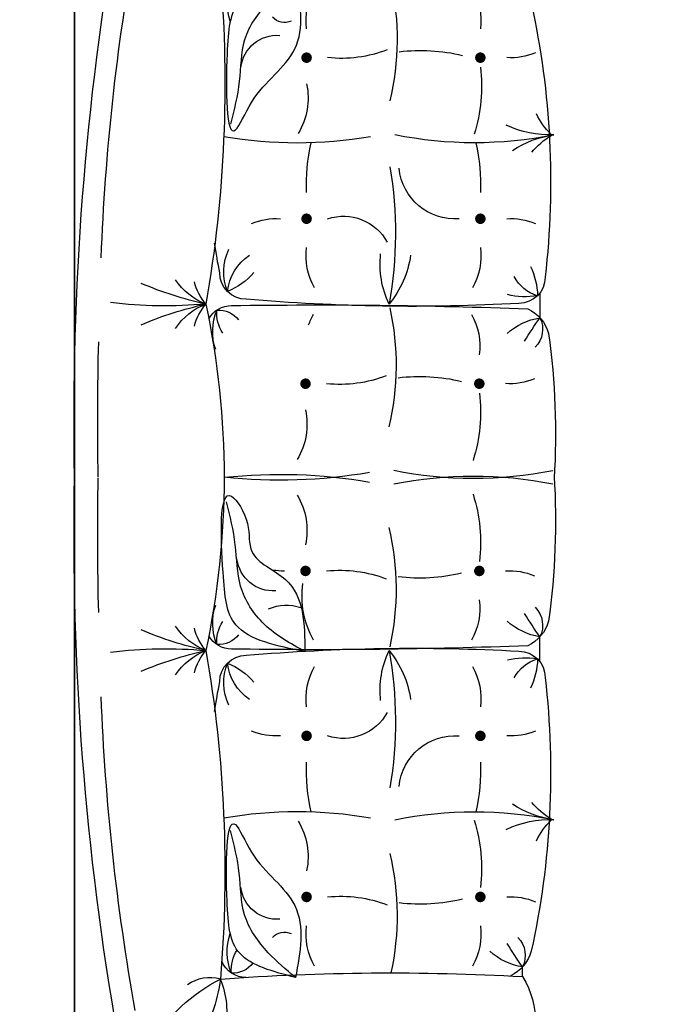
# Model space of a CAD drawing. Units: inches. Extents: x 844 to 2234, y 346 to 1084.
# Tile 7 of 93: x 1095 to 1114, y 680 to 710. Entities that reach past the tile are written whole.
import ezdxf

# ---------------------------------------------------------------- set-up
doc = ezdxf.new("R2010")
doc.units = ezdxf.units.IN
doc.header["$MEASUREMENT"] = 0
for name, color, linetype, lineweight in [('A-ANNO-DIMS', 2, 'Continuous', 18), ('A-WALL', 7, 'Continuous', 35), ('furniture', 8, 'Continuous', 18)]:
    doc.layers.add(name, color=color, linetype=linetype, lineweight=lineweight)
doc.layers.add('RA-AP-01$0$FURN', color=3, linetype='Continuous')
doc.layers.add('RA-AP-01$0$WOOD', color=64, linetype='Continuous')
doc.styles.get("Standard").update_dxf_attribs({"font": 'arial.ttf'})
doc.dimstyles.get("Standard").update_dxf_attribs({"dimtxt": 6, "dimasz": 3, "dimexe": 0.18, "dimexo": 0.0625, "dimgap": 0.09, "dimtad": 0, "dimtih": 1, "dimtoh": 1, "dimdec": 1, "dimzin": 0, "dimdsep": 46, "dimlunit": 3, "dimtxsty": 'Standard', "dimblk": 'ARCHTICK', "dimcen": 0.09, "dimadec": 0, "dimazin": 0, "dimtfac": 1, "dimtdec": 1, "dimtofl": 0, "dimtmove": 0, "dimatfit": 3, "dimfxl": 1, "dimtolj": 1, "dimtzin": 0, "dimarcsym": 0})

# ---------------------------------------------------------------- blocks, each defined once
blk = doc.blocks.new('A$C7EE91E48')
at = {"layer": 'RA-AP-01$0$FURN'}
for p, q in [((8.4752, -8.8836), (8.5044, -8.8836)), ((8.5044, -8.8836), (8.5227, -8.8836)), ((9.1476, -8.8836), (9.1292, -8.8836)), ((9.1768, -8.8836), (9.1476, -8.8836)), ((7.8765, -8.9166), (7.8948, -8.9166))]:
    blk.add_line(p, q, dxfattribs=at)
at = {"layer": 'RA-AP-01$0$FURN', "const_width": 0.01}
for points in [[(8.0279, -9.0019, -1), (8.0279, -8.9919, -1)], [(8.3342, -9.0019, 1), (8.3342, -8.9919, 1)], [(9.3177, -9.0019, -1), (9.3177, -8.9919, -1)], [(9.624, -9.0019, 1), (9.624, -8.9919, 1)], [(8.6479, -9.0039, -1), (8.6479, -8.9939, -1)], [(9.004, -9.0039, 1), (9.004, -8.9939, 1)], [(8.0279, -9.3223, 1), (8.0279, -9.3323, 1)], [(8.3342, -9.3223, -1), (8.3342, -9.3323, -1)], [(8.6479, -9.3243, 1), (8.6479, -9.3343, 1)], [(9.004, -9.3243, -1), (9.004, -9.3343, -1)], [(9.3177, -9.3223, 1), (9.3177, -9.3323, 1)], [(9.624, -9.3223, -1), (9.624, -9.3323, -1)]]:
    blk.add_lwpolyline(points, format="xyb", close=True, dxfattribs=at)
at = {"layer": 'RA-AP-01$0$FURN'}
for centre, radius, start, end in [((8.744, -10.2748), 1.4207, 86.5948, 97.7424), ((8.9079, -10.2748), 1.4207, 82.2576, 93.4052), ((8.2641, -10.4424), 1.5791, 83.4116, 102.408), ((8.0633, -8.7497), 0.1579, 296.9155, 314.5948), ((7.9834, -8.8653), 0.1916, 334.4169, 2.4147), ((7.4244, -9.0082), 0.7655, 348.5826, 11.3727), ((8.3595, -8.8326), 0.1864, 187.6182, 213.7074), ((8.3098, -8.7788), 0.1579, 211.9342, 229.6135), ((8.4452, -8.9237), 0.05, 0, 90), ((8.5734, -8.9396), 0.0754, 106.0166, 154.1254), ((8.0629, -9.0102), 0.7655, 348.5826, 11.3727), ((9.589, -9.0102), 0.7655, 168.6273, 191.4174), ((9.0785, -8.9396), 0.0754, 25.8746, 73.9834), ((9.2067, -8.9237), 0.05, 90, 180), ((9.3879, -10.4424), 1.5791, 77.592, 96.5884), ((9.3421, -8.7788), 0.1579, 310.3865, 328.0658), ((9.2924, -8.8326), 0.1864, 326.2926, 352.3818), ((10.2276, -9.0082), 0.7655, 168.6273, 191.4174), ((9.6686, -8.8653), 0.1916, 177.5853, 205.5831), ((9.5886, -8.7497), 0.1579, 225.4052, 243.0845), ((7.7865, -9.0661), 0.1745, 58.9518, 121.0482), ((7.9069, -8.939), 0.1213, 356.2685, 22.6624), ((8.4553, -8.939), 0.1213, 157.3376, 183.7315), ((8.4834, -9.0206), 0.1324, 91.1993, 116.1112), ((8.411, -8.8679), 0.0726, 297.3225, 343.6441), ((8.3504, -8.912), 0.1324, 345.3922, 10.3041), ((8.5446, -8.9264), 0.0479, 44.5975, 117.1929), ((8.6431, -8.8646), 0.1219, 188.9538, 221.9624), ((9.1542, -7.9707), 1.1102, 235.3335, 238.0671), ((8.5269, -8.941), 0.1213, 356.2685, 22.6624), ((9.1251, -8.941), 0.1213, 157.3376, 183.7315), ((9.1073, -8.9264), 0.0479, 62.8071, 135.4025), ((8.4977, -7.9707), 1.1102, 301.9329, 304.6665), ((9.0089, -8.8646), 0.1219, 318.0376, 351.0462), ((9.3016, -8.912), 0.1324, 169.6959, 194.6078), ((9.1686, -9.0206), 0.1324, 63.8888, 88.8007), ((9.241, -8.8679), 0.0726, 196.3559, 242.6775), ((9.1967, -8.939), 0.1213, 356.2685, 22.6624), ((9.7451, -8.939), 0.1213, 157.3376, 183.7315), ((7.9455, -8.9726), 0.0754, 106.0166, 154.1254), ((7.9168, -8.9594), 0.0479, 44.5975, 117.1929), ((19.2274, -9.306), 10.7293, 177.86728, 180.87576), ((-1.5755, -9.306), 10.7293, 359.12424, 2.13272), ((3.4096, -9.1677), 4.4739, 355.8523, 3.2171), ((8.0152, -8.8976), 0.1219, 188.9538, 221.9624), ((8.5263, -8.0037), 1.1102, 235.3335, 238.0671), ((4.8029, -9.1271), 3.698, 355.1082, 3.1536), ((12.8491, -9.1271), 3.698, 176.8464, 184.8918), ((7.9567, -9.1172), 0.1214, 82.3083, 119.8581), ((8.0823, -9.2969), 0.3024, 72.4119, 96.9055), ((8.2692, -9.3452), 0.3487, 87.5342, 103.1608), ((8.4055, -9.1172), 0.1214, 60.1419, 97.6917), ((8.5767, -9.1192), 0.1214, 82.3083, 119.8581), ((8.7023, -9.299), 0.3024, 72.4119, 96.9055), ((8.9496, -9.299), 0.3024, 83.0945, 107.5881), ((9.0753, -9.1192), 0.1214, 60.1419, 97.6917), ((9.2465, -9.1172), 0.1214, 82.3083, 119.8581), ((9.3827, -9.3452), 0.3487, 76.8392, 92.4658), ((9.5696, -9.2969), 0.3024, 83.0945, 107.5881), ((9.6953, -9.1172), 0.1214, 60.1419, 97.6917), ((8.3659, -9.111), 0.3517, 166.8325, 186.5875), ((8.2285, -9.0458), 0.106, 275.1859, 4.8073), ((8.9859, -9.113), 0.3517, 166.8325, 186.5875), ((8.666, -9.113), 0.3517, 353.4125, 13.1675), ((9.4234, -9.0458), 0.106, 175.1927, 264.8141), ((9.286, -9.111), 0.3517, 353.4125, 13.1675), ((8.378, -9.3133), 0.1855, 50.3168, 82.0523), ((9.2739, -9.3133), 0.1855, 97.9477, 129.6832), ((7.9929, -9.6653), 0.5101, 76.6878, 102.3818), ((9.6591, -9.6653), 0.5101, 77.6182, 103.3122), ((7.785, -9.2618), 0.2442, 354.0076, 21.0983), ((8.3614, -9.9068), 0.7485, 79.6011, 99.6906), ((8.4248, -9.2574), 0.0954, 118.8034, 198.2253), ((8.4207, -9.0107), 0.1769, 263.6796, 295.3608), ((8.6129, -9.6673), 0.5101, 76.6878, 102.3818), ((9.0391, -9.6673), 0.5101, 77.6182, 103.3122), ((9.2906, -9.9068), 0.7485, 80.3094, 100.3989), ((9.2312, -9.0107), 0.1769, 244.6392, 276.3204), ((9.2271, -9.2574), 0.0954, 341.7747, 61.1966), ((9.8669, -9.2618), 0.2442, 158.9017, 185.9924), ((8.405, -9.2638), 0.2442, 354.0076, 21.0983), ((9.2469, -9.2638), 0.2442, 158.9017, 185.9924), ((7.367, -9.3453), 0.8233, 350.2449, 9.7551), ((7.8327, -9.3782), 0.9989, 353.9343, 9.823), ((9.8193, -9.3782), 0.9989, 170.177, 186.0657), ((10.285, -9.3453), 0.8233, 170.2449, 189.7551), ((7.9567, -9.2069), 0.1214, 240.1419, 277.6917), ((8.1048, -9.4539), 0.1295, 58.6204, 102.0099), ((8.2692, -8.9789), 0.3487, 256.8392, 272.4658), ((8.4055, -9.2069), 0.1214, 262.3083, 299.8581), ((8.6002, -9.1634), 0.1726, 240.9024, 278.0073), ((9.0753, -9.209), 0.1214, 289.6086, 299.8581), ((9.2465, -9.2069), 0.1214, 240.1419, 277.6917), ((9.3827, -8.9789), 0.3487, 267.5342, 283.1608), ((9.5471, -9.4539), 0.1295, 77.9901, 121.3796), ((9.6953, -9.2069), 0.1214, 262.3083, 299.8581), ((8.5004, -9.3657), 0.0825, 335.8161, 19.2747), ((8.7248, -9.456), 0.1295, 58.6204, 102.0099), ((8.9271, -9.456), 0.1295, 77.9901, 121.3796), ((7.93, -9.3692), 0.031, 312.6211, 24.224), ((9.722, -9.3692), 0.031, 155.776, 227.3789), ((8.0543, -9.3837), 0.0689, 175.5384, 263.5805), ((8.4553, -9.3851), 0.1213, 176.2685, 202.6624), ((8.405, -9.3948), 0.2442, 0.7304, 5.9924), ((9.1967, -9.3851), 0.1213, 337.3376, 3.7315), ((9.5977, -9.3837), 0.0689, 276.4195, 4.4616), ((8.6789, -9.3912), 0.0689, 175.5384, 263.5805), ((7.9309, -9.4673), 0.0479, 127.3166, 183.4247), ((8.4847, -9.3794), 0.0991, 214.8912, 263.0774), ((8.3451, -9.5317), 0.1386, 22.9132, 48.7711), ((9.3068, -9.5317), 0.1386, 131.2289, 157.0868), ((9.1673, -9.3794), 0.0991, 276.9226, 325.1088), ((7.9247, -9.4424), 0.05, 180, 247.4173), ((8.4374, -9.4424), 0.05, 270, 0), ((9.2146, -9.4424), 0.05, 180, 270), ((7.8894, -9.4022), 0.0683, 264.7816, 303.327), ((7.9236, -9.3742), 0.1042, 247.1307, 289.5172), ((8.5494, -9.4699), 0.05, 180, 239.8522), ((8.5556, -9.4948), 0.0479, 127.3166, 183.4247), ((9.0963, -9.4948), 0.0479, 356.5753, 52.6834), ((9.1025, -9.4699), 0.05, 300.1478, 360), ((9.7283, -9.3742), 0.1042, 250.4828, 292.8693), ((7.5711, -9.3365), 0.3382, 301.7436, 332.7697), ((7.9152, -9.8125), 0.3242, 97.6974, 120.7014), ((7.8086, -9.649), 0.1699, 68.1488, 101.1222), ((7.8044, -9.5117), 0.0705, 323.5874, 16.8661), ((8.0772, -11.9348), 2.4522, 80.1542, 94.8039), ((8.1811, -8.1864), 1.3309, 278.6229, 281.1036), ((8.4354, -9.3857), 0.0993, 244.3656, 292.0953), ((8.8331, -11.1187), 1.6349, 90.2483, 101.88), ((8.514, -9.4297), 0.0683, 264.7816, 303.327), ((8.8189, -11.1187), 1.6349, 78.12, 89.7517), ((9.1379, -9.4297), 0.0683, 236.673, 275.2184), ((9.5748, -11.9348), 2.4522, 85.1961, 99.8458), ((9.2166, -9.3857), 0.0993, 247.9047, 295.6344), ((9.4709, -8.1864), 1.3309, 258.8964, 261.3771), ((8.5483, -9.4017), 0.1042, 247.1307, 289.5172), ((9.1036, -9.4017), 0.1042, 250.4828, 292.8693), ((8.3825, -9.4751), 0.122, 303.7136, 339.041), ((8.4279, -9.4377), 0.1062, 284.3648, 310.2303), ((7.8141, -9.3689), 0.6986, 337.0091, 347.612), ((7.6413, -9.5958), 0.8587, 353.0376, 5.1445), ((8.6105, -9.4751), 0.122, 200.959, 236.2864), ((8.5651, -9.4377), 0.1062, 229.7697, 255.6352), ((9.1788, -9.3689), 0.6986, 192.388, 202.9909), ((9.0415, -9.4751), 0.122, 303.7136, 339.041), ((9.0869, -9.4377), 0.1062, 284.3648, 310.2303), ((8.4731, -9.3689), 0.6986, 337.0091, 347.612), ((10.0107, -9.5958), 0.8587, 174.8555, 186.9624), ((9.2694, -9.4751), 0.122, 200.959, 236.2864), ((9.224, -9.4377), 0.1062, 229.7697, 255.6352), ((9.8378, -9.3689), 0.6986, 192.388, 202.9909), ((8.5724, -5.4361), 4.2848, 259.7801, 267.8084), ((9.0796, -5.4361), 4.2848, 272.1916, 280.2199), ((8.7159, -4.2841), 5.4854, 259.9939, 271.1496), ((8.936, -4.2841), 5.4854, 268.8504, 280.0061), ((8.7159, -4.2841), 5.4404, 268.4485, 271.1496), ((8.936, -4.2841), 5.4404, 268.8504, 271.5515)]:
    blk.add_arc(centre, radius, start, end, dxfattribs=at)
for points, knots in [([(7.8747, -9.3485), (7.9231, -9.3393), (7.9933, -9.326), (8.0638, -9.3901), (8.1031, -9.4315), (8.221, -9.4812), (8.0194, -9.4811), (7.9064, -9.4702), (7.8857, -9.3906), (7.8747, -9.3485)], [0, 0, 0, 0, 0.1367587, 0.1981302, 0.267773, 0.3281195, 0.4737578, 0.5765194, 0.6920332, 0.6920332, 0.6920332, 0.6920332]), ([(8.4947, -9.3305), (8.5098, -9.3579), (8.5387, -9.4102), (8.6151, -9.4603), (8.6994, -9.4595), (8.7521, -9.4728), (8.7791, -9.4797)], [0, 0, 0, 0, 0.0929945, 0.178054, 0.2574251, 0.3407808, 0.3407808, 0.3407808, 0.3407808]), ([(8.4947, -9.3305), (8.547, -9.3311), (8.63, -9.3319), (8.67, -9.4425), (8.7389, -9.4316), (8.8424, -9.4963), (8.6448, -9.4874), (8.5233, -9.4759), (8.5051, -9.3838), (8.4947, -9.3305)], [0, 0, 0, 0, 0.1415752, 0.2249019, 0.2789443, 0.3392908, 0.4849291, 0.5876907, 0.7285367, 0.7285367, 0.7285367, 0.7285367]), ([(9.7773, -9.3485), (9.7288, -9.3393), (9.6586, -9.326), (9.5882, -9.3901), (9.5488, -9.4315), (9.4309, -9.4812), (9.6325, -9.4811), (9.7455, -9.4702), (9.7663, -9.3906), (9.7773, -9.3485)], [0, 0, 0, 0, 0.1367587, 0.1981302, 0.267773, 0.3281195, 0.4737578, 0.5765194, 0.6920332, 0.6920332, 0.6920332, 0.6920332]), ([(7.8747, -9.3485), (7.8896, -9.3663), (7.9228, -9.4056), (7.9899, -9.4532), (8.0749, -9.4519), (8.1275, -9.4653), (8.1544, -9.4722)], [0, 0, 0, 0, 0.0700185, 0.155078, 0.2344492, 0.3178049, 0.3178049, 0.3178049, 0.3178049]), ([(9.7773, -9.3485), (9.7623, -9.3663), (9.7292, -9.4056), (9.662, -9.4532), (9.577, -9.4519), (9.5245, -9.4653), (9.4975, -9.4722)], [0, 0, 0, 0, 0.0700185, 0.155078, 0.2344492, 0.3178049, 0.3178049, 0.3178049, 0.3178049])]:
    blk.add_open_spline(points, degree=3, knots=knots, dxfattribs=at)
blk = doc.blocks.new('A$C5D2F253E')
at = {"layer": 'RA-AP-01$0$WOOD', "xscale": -1, "rotation": 180}
blk.add_blockref('A$C7EE91E48', (-8.833, -7.2888), dxfattribs=at)
blk = doc.blocks.new('_ArchTick')
at = {"color": 0, "linetype": 'ByBlock', "const_width": 0.15}
blk.add_lwpolyline([(-0.5, -0.5), (0.5, 0.5)], dxfattribs=at)
blk = doc.blocks.new('*D144')
at = {"layer": 'A-ANNO-DIMS', "color": 0, "lineweight": -2, "transparency": 16777216}
for p, q in [((1096.616, 439.373), (1096.616, 1074.743)), ((1143.116, 492.373), (1143.116, 1074.743)), ((1096.616, 1074.563), (1102.482, 1074.563)), ((1143.116, 1074.563), (1137.25, 1074.563))]:
    blk.add_line(p, q, dxfattribs=at)
at = {"layer": 'Defpoints', "color": 0, "transparency": 16777216}
for p in [(1143.116, 1074.563), (1143.116, 492.311), (1096.616, 439.311)]:
    blk.add_point(p, dxfattribs=at)
at = {"layer": 'A-ANNO-DIMS', "color": 0, "lineweight": -2, "transparency": 16777216, "xscale": 3, "yscale": 3, "zscale": 3, "rotation": 180}
blk.add_blockref('_ArchTick', (1096.616, 1074.563), dxfattribs=at)
at = {"layer": 'A-ANNO-DIMS', "color": 0, "lineweight": -2, "transparency": 16777216, "xscale": 3, "yscale": 3, "zscale": 3}
blk.add_blockref('_ArchTick', (1143.116, 1074.563), dxfattribs=at)
at = {"layer": 'A-ANNO-DIMS', "color": 0, "transparency": 16777216, "insert": (1119.866, 1074.563), "char_height": 6, "attachment_point": 5}
blk.add_mtext('\\A1;3\'-10 1/2"', dxfattribs=at)

msp = doc.modelspace()

# ---------------------------------------------------------------- linework, layer by layer
at = {"layer": 'A-WALL'}
msp.add_line((1096.616, 761.311), (1096.616, 624.311), dxfattribs=at)

# ---------------------------------------------------------------- block references
at = {"layer": 'furniture', "xscale": 15.94108302203742, "yscale": 15.94108302203742, "zscale": 15.94108302203742, "rotation": 90}
msp.add_blockref('A$C5D2F253E', (1136.148, 696.258), dxfattribs=at)

# ---------------------------------------------------------------- dimensions: what is measured, and where the dimension line sits
at = {"layer": 'A-ANNO-DIMS'}
dim = msp.add_linear_dim(base=(1143.116, 1074.563), p1=(1096.616, 439.311), p2=(1143.116, 492.311), dimstyle='Standard', override={"dimdec": 1, "dimlfac": 1, "dimrnd": 0, "dimzin": 1, "dimdsep": 46, "dimlunit": 4, "dimfrac": 2}, dxfattribs=at)
dim.commit()
dim.dimension.update_dxf_attribs({"geometry": '*D144', "text_midpoint": (1119.866, 1074.563)})

doc.saveas('drawing.dxf')
